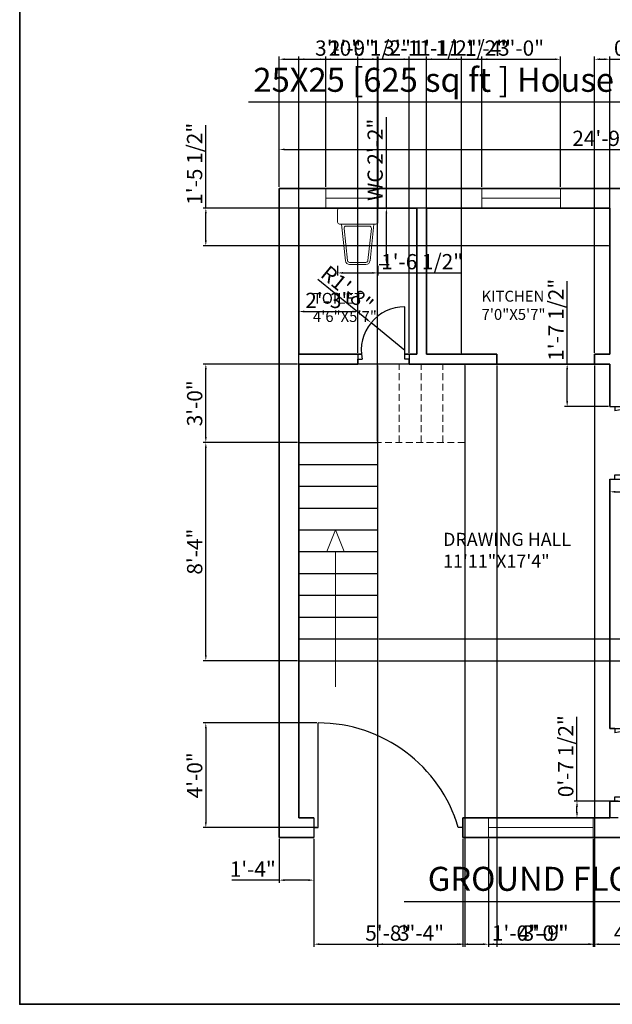
# Model space of a CAD drawing. Units: inches. Extents: x 1484 to 2008, y 1843 to 2590.
# Tile 1 of 21: x 1484 to 1756, y 1843 to 2295. Entities that reach past the tile are written whole.
import ezdxf

# ---------------------------------------------------------------- set-up
doc = ezdxf.new("R2010")
doc.units = ezdxf.units.IN
doc.linetypes.add('HIDDEN2', pattern=[4.7625, 3.175, -1.5875])
for name, color, linetype, lineweight in [('A-ANNO-DIMS', 2, 'Continuous', 18), ('A-ANNO-SYMB', 7, 'Continuous', 18), ('A-ANNO-TEXT', 7, 'Continuous', 25), ('A-ANNO-TTLB', 7, 'Continuous', 35), ('A-AREA-IDEN', 7, 'Continuous', 18), ('A-DOOR', 4, 'Continuous', 25), ('A-FLOR-FIXT', 9, 'Continuous', 18), ('A-FLOR-STRS', 7, 'Continuous', 25), ('A-FLOR-STRS-OVHD', 253, 'HIDDEN2', 18), ('A-GLAZ', 4, 'Continuous', 18), ('A-WALL', 7, 'Continuous', 35)]:
    doc.layers.add(name, color=color, linetype=linetype, lineweight=lineweight)
doc.styles.get("Standard").update_dxf_attribs({"font": 'arial.ttf'})
doc.dimstyles.new('ISO-25', dxfattribs={"dimtxt": 7, "dimasz": 2.5, "dimexe": 1.25, "dimexo": 0.625, "dimtad": 1, "dimdec": 0, "dimlunit": 3, "dimtxsty": 'Standard', "dimcen": 2.5, "dimadec": 0, "dimazin": 0, "dimtfac": 1, "dimtdec": 0, "dimtmove": 0, "dimatfit": 3, "dimfxl": 1, "dimarcsym": 0})

# ---------------------------------------------------------------- blocks, each defined once
blk = doc.blocks.new('A$C274B7A8C')
for p, q in [((0, 0.525), (0, 0.675)), ((0.025, 0.7), (0.475, 0.7)), ((0.5, 0.675), (0.5, 0.525)), ((0.475, 0.5), (0.025, 0.5)), ((0.05, 0.5), (0.098, 0.045)), ((0.402, 0.045), (0.45, 0.5)), ((0.081, 0.447), (0.123, 0.047)), ((0.106, 0.475), (0.394, 0.475)), ((0.377, 0.047), (0.419, 0.447)), ((0.148, 0.025), (0.352, 0.025)), ((0.148, 0), (0.352, 0))]:
    blk.add_line(p, q)
for centre, radius, start, end in [((0.025, 0.675), 0.025, 90, 180), ((0.475, 0.675), 0.025, 0, 90), ((0.025, 0.525), 0.025, 180, 270), ((0.475, 0.525), 0.025, 270, 0), ((0.106, 0.45), 0.025, 90, 186.009), ((0.394, 0.45), 0.025, 353.991, 90), ((0.148, 0.05), 0.05, 186.009, 270), ((0.148, 0.05), 0.025, 186.009, 270), ((0.352, 0.05), 0.025, 270, 353.991), ((0.352, 0.05), 0.05, 270, 353.991)]:
    blk.add_arc(centre, radius, start, end)
blk = doc.blocks.new('*D2')
at = {"layer": 'A-ANNO-DIMS', "color": 0, "lineweight": -2, "transparency": 16777216}
for p, q in [((1602.92, 2217.93), (1602.92, 2236.39)), ((1605.42, 2235.14), (1897.42, 2235.14)), ((1899.92, 2217.93), (1899.92, 2236.39))]:
    blk.add_line(p, q, dxfattribs=at)
at = {"layer": 'A-ANNO-DIMS', "color": 0, "transparency": 16777216}
for points in [[(1605.42, 2235.55), (1605.42, 2234.72), (1602.92, 2235.14)], [(1897.42, 2235.55), (1897.42, 2234.72), (1899.92, 2235.14)]]:
    blk.add_solid(points, dxfattribs=at)
at = {"layer": 'Defpoints', "color": 0, "transparency": 16777216}
for p in [(1899.92, 2235.14), (1602.92, 2217.3), (1899.92, 2217.3)]:
    blk.add_point(p, dxfattribs=at)
at = {"layer": 'A-ANNO-DIMS', "color": 0, "transparency": 16777216, "insert": (1750.41, 2239.33), "char_height": 7, "attachment_point": 5}
blk.add_mtext('24\'-9"', dxfattribs=at)
blk = doc.blocks.new('DOOR-SWING-36IN')
for p, q in [((-2.25, 31.33), (2.25, 31.33)), ((0, 31.33), (0, 29.33)), ((-2.25, -2), (2.25, -2)), ((0, -2), (0, 0)), ((0, 0), (36, 0))]:
    blk.add_line(p, q)
blk.add_arc((6.05, 0), 29.95, 0, 101.6643)
blk = doc.blocks.new('*D11')
at = {"layer": 'A-ANNO-DIMS', "color": 0, "lineweight": -2, "transparency": 16777216}
for p, q in [((1754.42, 2083.34), (1754.42, 2076.98)), ((1792.67, 2083.34), (1792.67, 2076.98)), ((1756.92, 2078.23), (1790.17, 2078.23)), ((1792.67, 2078.23), (1887.1, 2078.23))]:
    blk.add_line(p, q, dxfattribs=at)
at = {"layer": 'A-ANNO-DIMS', "color": 0, "transparency": 16777216}
for points in [[(1756.92, 2078.64), (1756.92, 2077.81), (1754.42, 2078.23)], [(1790.17, 2078.64), (1790.17, 2077.81), (1792.67, 2078.23)]]:
    blk.add_solid(points, dxfattribs=at)
at = {"layer": 'Defpoints', "color": 0, "transparency": 16777216}
for p in [(1754.42, 2083.96), (1792.67, 2083.96), (1792.67, 2078.23)]:
    blk.add_point(p, dxfattribs=at)
at = {"layer": 'A-ANNO-DIMS', "color": 0, "transparency": 16777216, "insert": (1841.14, 2082.47), "char_height": 7, "attachment_point": 5}
blk.add_mtext('DOOR 3\'-2 1/2" TYP.', dxfattribs=at)
blk = doc.blocks.new('*D17')
at = {"layer": 'A-ANNO-DIMS', "color": 0, "lineweight": -2, "transparency": 16777216}
for p, q in [((1652.04, 2208.3), (1652.04, 2249.96)), ((1648.78, 2208.3), (1653.29, 2208.3)), ((1652.04, 2184.93), (1652.04, 2205.8)), ((1648.78, 2182.43), (1653.29, 2182.43))]:
    blk.add_line(p, q, dxfattribs=at)
at = {"layer": 'A-ANNO-DIMS', "color": 0, "transparency": 16777216}
for points in [[(1651.62, 2205.8), (1652.46, 2205.8), (1652.04, 2208.3)], [(1651.62, 2184.93), (1652.46, 2184.93), (1652.04, 2182.43)]]:
    blk.add_solid(points, dxfattribs=at)
at = {"layer": 'Defpoints', "color": 0, "transparency": 16777216}
for p in [(1648.16, 2208.3), (1652.04, 2208.3), (1648.16, 2182.43)]:
    blk.add_point(p, dxfattribs=at)
at = {"layer": 'A-ANNO-DIMS', "color": 0, "transparency": 16777216, "insert": (1647.8, 2230.38), "char_height": 7, "attachment_point": 5, "rotation": 90}
blk.add_mtext('WC 2\'-2"', dxfattribs=at)
blk = doc.blocks.new('*D18')
at = {"layer": 'A-ANNO-DIMS', "color": 0, "lineweight": -2, "transparency": 16777216}
for p, q in [((1629.68, 2181.81), (1629.68, 2177.3)), ((1648.16, 2181.81), (1648.16, 2177.3)), ((1632.18, 2178.55), (1645.66, 2178.55)), ((1648.16, 2178.55), (1686.17, 2178.55))]:
    blk.add_line(p, q, dxfattribs=at)
at = {"layer": 'A-ANNO-DIMS', "color": 0, "transparency": 16777216}
for points in [[(1632.18, 2178.97), (1632.18, 2178.13), (1629.68, 2178.55)], [(1645.66, 2178.97), (1645.66, 2178.13), (1648.16, 2178.55)]]:
    blk.add_solid(points, dxfattribs=at)
at = {"layer": 'Defpoints', "color": 0, "transparency": 16777216}
for p in [(1629.68, 2182.43), (1648.16, 2182.43), (1648.16, 2178.55)]:
    blk.add_point(p, dxfattribs=at)
at = {"layer": 'A-ANNO-DIMS', "color": 0, "transparency": 16777216, "insert": (1668.41, 2182.79), "char_height": 7, "attachment_point": 5}
blk.add_mtext('1\'-6 1/2"', dxfattribs=at)
blk = doc.blocks.new('*D19')
at = {"layer": 'A-ANNO-DIMS', "color": 0, "lineweight": -2, "transparency": 16777216}
for p, q in [((1602.92, 1919.18), (1602.92, 1899)), ((1618.8, 1919.18), (1618.8, 1899)), ((1602.92, 1900.25), (1581.22, 1900.25)), ((1616.3, 1900.25), (1605.42, 1900.25))]:
    blk.add_line(p, q, dxfattribs=at)
at = {"layer": 'A-ANNO-DIMS', "color": 0, "transparency": 16777216}
for points in [[(1605.42, 1900.67), (1605.42, 1899.84), (1602.92, 1900.25)], [(1616.3, 1900.67), (1616.3, 1899.84), (1618.8, 1900.25)]]:
    blk.add_solid(points, dxfattribs=at)
at = {"layer": 'Defpoints', "color": 0, "transparency": 16777216}
for p in [(1602.92, 1919.8), (1618.8, 1919.8), (1602.92, 1900.25)]:
    blk.add_point(p, dxfattribs=at)
at = {"layer": 'A-ANNO-DIMS', "color": 0, "transparency": 16777216, "insert": (1590.82, 1904.39), "char_height": 7, "attachment_point": 5}
blk.add_mtext('1\'-4"', dxfattribs=at)
blk = doc.blocks.new('*D20')
at = {"layer": 'A-ANNO-DIMS', "color": 0, "lineweight": -2, "transparency": 16777216}
for p, q in [((1618.8, 1919.18), (1618.8, 1869.63)), ((1686.99, 1919.18), (1686.99, 1869.63)), ((1621.3, 1870.88), (1684.49, 1870.88))]:
    blk.add_line(p, q, dxfattribs=at)
at = {"layer": 'A-ANNO-DIMS', "color": 0, "transparency": 16777216}
for points in [[(1621.3, 1871.3), (1621.3, 1870.46), (1618.8, 1870.88)], [(1684.49, 1871.3), (1684.49, 1870.46), (1686.99, 1870.88)]]:
    blk.add_solid(points, dxfattribs=at)
at = {"layer": 'Defpoints', "color": 0, "transparency": 16777216}
for p in [(1618.8, 1919.8), (1686.99, 1919.8), (1686.99, 1870.88)]:
    blk.add_point(p, dxfattribs=at)
at = {"layer": 'A-ANNO-DIMS', "color": 0, "transparency": 16777216, "insert": (1652.89, 1875.08), "char_height": 7, "attachment_point": 5}
blk.add_mtext('5\'-8"', dxfattribs=at)
blk = doc.blocks.new('*D21')
at = {"layer": 'A-ANNO-DIMS', "color": 0, "lineweight": -2, "transparency": 16777216}
for p, q in [((1686.99, 1919.18), (1686.99, 1869.63)), ((1698.84, 1919.18), (1698.84, 1869.63)), ((1689.49, 1870.88), (1696.34, 1870.88)), ((1698.84, 1870.88), (1720.54, 1870.88))]:
    blk.add_line(p, q, dxfattribs=at)
at = {"layer": 'A-ANNO-DIMS', "color": 0, "transparency": 16777216}
for points in [[(1689.49, 1871.3), (1689.49, 1870.46), (1686.99, 1870.88)], [(1696.34, 1871.3), (1696.34, 1870.46), (1698.84, 1870.88)]]:
    blk.add_solid(points, dxfattribs=at)
at = {"layer": 'Defpoints', "color": 0, "transparency": 16777216}
for p in [(1686.99, 1919.8), (1698.84, 1919.8), (1698.84, 1870.88)]:
    blk.add_point(p, dxfattribs=at)
at = {"layer": 'A-ANNO-DIMS', "color": 0, "transparency": 16777216, "insert": (1710.94, 1875.08), "char_height": 7, "attachment_point": 5}
blk.add_mtext('1\'-0"', dxfattribs=at)
blk = doc.blocks.new('*D22')
at = {"layer": 'A-ANNO-DIMS', "color": 0, "lineweight": -2, "transparency": 16777216}
for p, q in [((1698.84, 1919.18), (1698.84, 1869.63)), ((1746.84, 1919.18), (1746.84, 1869.63)), ((1701.34, 1870.88), (1744.34, 1870.88))]:
    blk.add_line(p, q, dxfattribs=at)
at = {"layer": 'A-ANNO-DIMS', "color": 0, "transparency": 16777216}
for points in [[(1701.34, 1871.3), (1701.34, 1870.46), (1698.84, 1870.88)], [(1744.34, 1871.3), (1744.34, 1870.46), (1746.84, 1870.88)]]:
    blk.add_solid(points, dxfattribs=at)
at = {"layer": 'Defpoints', "color": 0, "transparency": 16777216}
for p in [(1698.84, 1919.8), (1746.84, 1919.8), (1746.84, 1870.88)]:
    blk.add_point(p, dxfattribs=at)
at = {"layer": 'A-ANNO-DIMS', "color": 0, "transparency": 16777216, "insert": (1722.84, 1875.08), "char_height": 7, "attachment_point": 5}
blk.add_mtext('4\'-0"', dxfattribs=at)
blk = doc.blocks.new('*D23')
at = {"layer": 'A-ANNO-DIMS', "color": 0, "lineweight": -2, "transparency": 16777216}
for p, q in [((1746.84, 1919.18), (1746.84, 1869.63)), ((1803.22, 1919.18), (1803.22, 1869.63)), ((1749.34, 1870.88), (1800.72, 1870.88))]:
    blk.add_line(p, q, dxfattribs=at)
at = {"layer": 'A-ANNO-DIMS', "color": 0, "transparency": 16777216}
for points in [[(1749.34, 1871.3), (1749.34, 1870.46), (1746.84, 1870.88)], [(1800.72, 1871.3), (1800.72, 1870.46), (1803.22, 1870.88)]]:
    blk.add_solid(points, dxfattribs=at)
at = {"layer": 'Defpoints', "color": 0, "transparency": 16777216}
for p in [(1746.84, 1919.8), (1803.22, 1919.8), (1803.22, 1870.88)]:
    blk.add_point(p, dxfattribs=at)
at = {"layer": 'A-ANNO-DIMS', "color": 0, "transparency": 16777216, "insert": (1775.03, 1875.12), "char_height": 7, "attachment_point": 5}
blk.add_mtext('4\'-8 1/2"', dxfattribs=at)
blk = doc.blocks.new('*D24')
at = {"layer": 'A-ANNO-DIMS', "color": 0, "lineweight": -2, "transparency": 16777216}
for p, q in [((1602.92, 2217.93), (1602.92, 2277.72)), ((1605.42, 2276.47), (1621.73, 2276.47)), ((1624.23, 2217.93), (1624.23, 2277.72)), ((1624.23, 2276.47), (1662.24, 2276.47))]:
    blk.add_line(p, q, dxfattribs=at)
at = {"layer": 'A-ANNO-DIMS', "color": 0, "transparency": 16777216}
for points in [[(1605.42, 2276.89), (1605.42, 2276.06), (1602.92, 2276.47)], [(1621.73, 2276.89), (1621.73, 2276.06), (1624.23, 2276.47)]]:
    blk.add_solid(points, dxfattribs=at)
at = {"layer": 'Defpoints', "color": 0, "transparency": 16777216}
for p in [(1624.23, 2276.47), (1602.92, 2217.3), (1624.23, 2217.3)]:
    blk.add_point(p, dxfattribs=at)
at = {"layer": 'A-ANNO-DIMS', "color": 0, "transparency": 16777216, "insert": (1644.48, 2280.72), "char_height": 7, "attachment_point": 5}
blk.add_mtext('1\'-9 1/2"', dxfattribs=at)
blk = doc.blocks.new('*D25')
at = {"layer": 'A-ANNO-DIMS', "color": 0, "lineweight": -2, "transparency": 16777216}
for p, q in [((1624.23, 2217.93), (1624.23, 2277.72)), ((1626.73, 2276.47), (1645.73, 2276.47)), ((1648.23, 2217.93), (1648.23, 2277.72))]:
    blk.add_line(p, q, dxfattribs=at)
at = {"layer": 'A-ANNO-DIMS', "color": 0, "transparency": 16777216}
for points in [[(1626.73, 2276.89), (1626.73, 2276.06), (1624.23, 2276.47)], [(1645.73, 2276.89), (1645.73, 2276.06), (1648.23, 2276.47)]]:
    blk.add_solid(points, dxfattribs=at)
at = {"layer": 'Defpoints', "color": 0, "transparency": 16777216}
for p in [(1648.23, 2276.47), (1624.23, 2217.3), (1648.23, 2217.3)]:
    blk.add_point(p, dxfattribs=at)
at = {"layer": 'A-ANNO-DIMS', "color": 0, "transparency": 16777216, "insert": (1636.23, 2280.67), "char_height": 7, "attachment_point": 5}
blk.add_mtext('2\'-0"', dxfattribs=at)
blk = doc.blocks.new('*D26')
at = {"layer": 'A-ANNO-DIMS', "color": 0, "lineweight": -2, "transparency": 16777216}
for p, q in [((1648.23, 2217.93), (1648.23, 2277.72)), ((1650.73, 2276.47), (1693.24, 2276.47)), ((1695.74, 2217.93), (1695.74, 2277.72))]:
    blk.add_line(p, q, dxfattribs=at)
at = {"layer": 'A-ANNO-DIMS', "color": 0, "transparency": 16777216}
for points in [[(1650.73, 2276.89), (1650.73, 2276.06), (1648.23, 2276.47)], [(1693.24, 2276.89), (1693.24, 2276.06), (1695.74, 2276.47)]]:
    blk.add_solid(points, dxfattribs=at)
at = {"layer": 'Defpoints', "color": 0, "transparency": 16777216}
for p in [(1695.74, 2276.47), (1648.23, 2217.3), (1695.74, 2217.3)]:
    blk.add_point(p, dxfattribs=at)
at = {"layer": 'A-ANNO-DIMS', "color": 0, "transparency": 16777216, "insert": (1671.98, 2280.72), "char_height": 7, "attachment_point": 5}
blk.add_mtext('3\'-11 1/2"', dxfattribs=at)
blk = doc.blocks.new('*D27')
at = {"layer": 'A-ANNO-DIMS', "color": 0, "lineweight": -2, "transparency": 16777216}
for p, q in [((1695.74, 2217.93), (1695.74, 2277.72)), ((1698.24, 2276.47), (1729.24, 2276.47)), ((1731.74, 2217.93), (1731.74, 2277.72))]:
    blk.add_line(p, q, dxfattribs=at)
at = {"layer": 'A-ANNO-DIMS', "color": 0, "transparency": 16777216}
for points in [[(1698.24, 2276.89), (1698.24, 2276.06), (1695.74, 2276.47)], [(1729.24, 2276.89), (1729.24, 2276.06), (1731.74, 2276.47)]]:
    blk.add_solid(points, dxfattribs=at)
at = {"layer": 'Defpoints', "color": 0, "transparency": 16777216}
for p in [(1731.74, 2276.47), (1695.74, 2217.3), (1731.74, 2217.3)]:
    blk.add_point(p, dxfattribs=at)
at = {"layer": 'A-ANNO-DIMS', "color": 0, "transparency": 16777216, "insert": (1713.74, 2280.68), "char_height": 7, "attachment_point": 5}
blk.add_mtext('3\'-0"', dxfattribs=at)
blk = doc.blocks.new('*D29')
at = {"layer": 'A-ANNO-DIMS', "color": 0, "lineweight": -2, "transparency": 16777216}
for p, q in [((1620.17, 1972.3), (1568.06, 1972.3)), ((1569.31, 1969.8), (1569.31, 1926.8)), ((1620.17, 1924.3), (1568.06, 1924.3))]:
    blk.add_line(p, q, dxfattribs=at)
at = {"layer": 'A-ANNO-DIMS', "color": 0, "transparency": 16777216}
for points in [[(1568.9, 1969.8), (1569.73, 1969.8), (1569.31, 1972.3)], [(1568.9, 1926.8), (1569.73, 1926.8), (1569.31, 1924.3)]]:
    blk.add_solid(points, dxfattribs=at)
at = {"layer": 'Defpoints', "color": 0, "transparency": 16777216}
for p in [(1620.8, 1972.3), (1569.31, 1924.3), (1620.8, 1924.3)]:
    blk.add_point(p, dxfattribs=at)
at = {"layer": 'A-ANNO-DIMS', "color": 0, "transparency": 16777216, "insert": (1565.11, 1948.3), "char_height": 7, "attachment_point": 5, "rotation": 90}
blk.add_mtext('4\'-0"', dxfattribs=at)
blk = doc.blocks.new('*D30')
at = {"layer": 'A-ANNO-DIMS', "color": 0, "lineweight": -2, "transparency": 16777216}
for p, q in [((1611.92, 2101.43), (1611.92, 2277.72)), ((1614.42, 2276.47), (1645.42, 2276.47)), ((1647.92, 2101.43), (1647.92, 2277.72))]:
    blk.add_line(p, q, dxfattribs=at)
at = {"layer": 'A-ANNO-DIMS', "color": 0, "transparency": 16777216}
for points in [[(1614.42, 2276.89), (1614.42, 2276.06), (1611.92, 2276.47)], [(1645.42, 2276.89), (1645.42, 2276.06), (1647.92, 2276.47)]]:
    blk.add_solid(points, dxfattribs=at)
at = {"layer": 'Defpoints', "color": 0, "transparency": 16777216}
for p in [(1647.92, 2276.47), (1611.92, 2100.8), (1647.92, 2100.8)]:
    blk.add_point(p, dxfattribs=at)
at = {"layer": 'A-ANNO-DIMS', "color": 0, "transparency": 16777216, "insert": (1629.92, 2280.68), "char_height": 7, "attachment_point": 5}
blk.add_mtext('3\'-0"', dxfattribs=at)
blk = doc.blocks.new('*D31')
at = {"layer": 'A-ANNO-DIMS', "color": 0, "lineweight": -2, "transparency": 16777216}
for p, q in [((1611.29, 2100.8), (1568.06, 2100.8)), ((1569.31, 2003.3), (1569.31, 2098.3)), ((1611.29, 2000.8), (1568.06, 2000.8))]:
    blk.add_line(p, q, dxfattribs=at)
at = {"layer": 'A-ANNO-DIMS', "color": 0, "transparency": 16777216}
for points in [[(1568.9, 2098.3), (1569.73, 2098.3), (1569.31, 2100.8)], [(1568.9, 2003.3), (1569.73, 2003.3), (1569.31, 2000.8)]]:
    blk.add_solid(points, dxfattribs=at)
at = {"layer": 'Defpoints', "color": 0, "transparency": 16777216}
for p in [(1569.31, 2100.8), (1611.92, 2100.8), (1611.92, 2000.8)]:
    blk.add_point(p, dxfattribs=at)
at = {"layer": 'A-ANNO-DIMS', "color": 0, "transparency": 16777216, "insert": (1565.11, 2050.8), "char_height": 7, "attachment_point": 5, "rotation": 90}
blk.add_mtext('8\'-4"', dxfattribs=at)
blk = doc.blocks.new('*D32')
at = {"layer": 'A-ANNO-DIMS', "color": 0, "lineweight": -2, "transparency": 16777216}
for p, q in [((1961.85, 2010.8), (1961.85, 2038.6)), ((1648.54, 2010.8), (1963.1, 2010.8)), ((1961.85, 2003.3), (1961.85, 2008.3)), ((1648.54, 2000.8), (1963.1, 2000.8))]:
    blk.add_line(p, q, dxfattribs=at)
at = {"layer": 'A-ANNO-DIMS', "color": 0, "transparency": 16777216}
for points in [[(1961.44, 2008.3), (1962.27, 2008.3), (1961.85, 2010.8)], [(1961.44, 2003.3), (1962.27, 2003.3), (1961.85, 2000.8)]]:
    blk.add_solid(points, dxfattribs=at)
at = {"layer": 'Defpoints', "color": 0, "transparency": 16777216}
for p in [(1647.92, 2010.8), (1961.85, 2010.8), (1647.92, 2000.8)]:
    blk.add_point(p, dxfattribs=at)
at = {"layer": 'A-ANNO-DIMS', "color": 0, "transparency": 16777216, "insert": (1957.66, 2025.95), "char_height": 7, "attachment_point": 5, "rotation": 90}
blk.add_mtext('0\'-10"', dxfattribs=at)
blk = doc.blocks.new('*D33')
at = {"layer": 'A-ANNO-DIMS', "color": 0, "lineweight": -2, "transparency": 16777216}
for p, q in [((1611.29, 2136.8), (1568.06, 2136.8)), ((1569.31, 2103.3), (1569.31, 2134.3)), ((1611.29, 2100.8), (1568.06, 2100.8))]:
    blk.add_line(p, q, dxfattribs=at)
at = {"layer": 'A-ANNO-DIMS', "color": 0, "transparency": 16777216}
for points in [[(1568.9, 2134.3), (1569.73, 2134.3), (1569.31, 2136.8)], [(1568.9, 2103.3), (1569.73, 2103.3), (1569.31, 2100.8)]]:
    blk.add_solid(points, dxfattribs=at)
at = {"layer": 'Defpoints', "color": 0, "transparency": 16777216}
for p in [(1569.31, 2136.8), (1611.92, 2136.8), (1611.92, 2100.8)]:
    blk.add_point(p, dxfattribs=at)
at = {"layer": 'A-ANNO-DIMS', "color": 0, "transparency": 16777216, "insert": (1565.11, 2118.8), "char_height": 7, "attachment_point": 5, "rotation": 90}
blk.add_mtext('3\'-0"', dxfattribs=at)
blk = doc.blocks.new('*D34')
at = {"layer": 'A-ANNO-DIMS', "color": 0, "lineweight": -2, "transparency": 16777216}
for p, q in [((1647.92, 2136.18), (1647.92, 1869.63)), ((1687.92, 2136.18), (1687.92, 1869.63)), ((1650.42, 1870.88), (1685.42, 1870.88))]:
    blk.add_line(p, q, dxfattribs=at)
at = {"layer": 'A-ANNO-DIMS', "color": 0, "transparency": 16777216}
for points in [[(1650.42, 1871.3), (1650.42, 1870.46), (1647.92, 1870.88)], [(1685.42, 1871.3), (1685.42, 1870.46), (1687.92, 1870.88)]]:
    blk.add_solid(points, dxfattribs=at)
at = {"layer": 'Defpoints', "color": 0, "transparency": 16777216}
for p in [(1647.92, 2136.8), (1687.92, 2136.8), (1687.92, 1870.88)]:
    blk.add_point(p, dxfattribs=at)
at = {"layer": 'A-ANNO-DIMS', "color": 0, "transparency": 16777216, "insert": (1667.92, 1875.08), "char_height": 7, "attachment_point": 5}
blk.add_mtext('3\'-4"', dxfattribs=at)
blk = doc.blocks.new('*D35')
at = {"layer": 'A-ANNO-DIMS', "color": 0, "lineweight": -2, "transparency": 16777216}
for p, q in [((1638.92, 2141.93), (1638.92, 2277.72)), ((1641.42, 2276.47), (1660.01, 2276.47)), ((1662.51, 2141.93), (1662.51, 2277.72)), ((1662.51, 2276.47), (1705.96, 2276.47))]:
    blk.add_line(p, q, dxfattribs=at)
at = {"layer": 'A-ANNO-DIMS', "color": 0, "transparency": 16777216}
for points in [[(1641.42, 2276.89), (1641.42, 2276.06), (1638.92, 2276.47)], [(1660.01, 2276.89), (1660.01, 2276.06), (1662.51, 2276.47)]]:
    blk.add_solid(points, dxfattribs=at)
at = {"layer": 'Defpoints', "color": 0, "transparency": 16777216}
for p in [(1662.51, 2276.47), (1638.92, 2141.3), (1662.51, 2141.3)]:
    blk.add_point(p, dxfattribs=at)
at = {"layer": 'A-ANNO-DIMS', "color": 0, "transparency": 16777216, "insert": (1685.48, 2280.72), "char_height": 7, "attachment_point": 5}
blk.add_mtext('1\'-11 1/2"', dxfattribs=at)
blk = doc.blocks.new('*D36')
at = {"layer": 'A-ANNO-DIMS', "color": 0, "lineweight": -2, "transparency": 16777216}
for p, q in [((1611.92, 2141.93), (1611.92, 2162.1)), ((1638.92, 2141.93), (1638.92, 2162.1)), ((1614.42, 2160.85), (1636.42, 2160.85))]:
    blk.add_line(p, q, dxfattribs=at)
at = {"layer": 'A-ANNO-DIMS', "color": 0, "transparency": 16777216}
for points in [[(1614.42, 2161.27), (1614.42, 2160.44), (1611.92, 2160.85)], [(1636.42, 2161.27), (1636.42, 2160.44), (1638.92, 2160.85)]]:
    blk.add_solid(points, dxfattribs=at)
at = {"layer": 'Defpoints', "color": 0, "transparency": 16777216}
for p in [(1638.92, 2160.85), (1611.92, 2141.3), (1638.92, 2141.3)]:
    blk.add_point(p, dxfattribs=at)
at = {"layer": 'A-ANNO-DIMS', "color": 0, "transparency": 16777216, "insert": (1625.42, 2165.05), "char_height": 7, "attachment_point": 5}
blk.add_mtext('2\'-3"', dxfattribs=at)
blk = doc.blocks.new('*D37')
at = {"layer": 'A-ANNO-DIMS', "color": 0, "lineweight": -2, "transparency": 16777216}
for p, q in [((1702.57, 2136.18), (1702.57, 1869.63)), ((1747.43, 2136.18), (1747.43, 1869.63)), ((1705.07, 1870.88), (1744.93, 1870.88))]:
    blk.add_line(p, q, dxfattribs=at)
at = {"layer": 'A-ANNO-DIMS', "color": 0, "transparency": 16777216}
for points in [[(1705.07, 1871.3), (1705.07, 1870.46), (1702.57, 1870.88)], [(1744.93, 1871.3), (1744.93, 1870.46), (1747.43, 1870.88)]]:
    blk.add_solid(points, dxfattribs=at)
at = {"layer": 'Defpoints', "color": 0, "transparency": 16777216}
for p in [(1702.57, 2136.8), (1747.43, 2136.8), (1747.43, 1870.88)]:
    blk.add_point(p, dxfattribs=at)
at = {"layer": 'A-ANNO-DIMS', "color": 0, "transparency": 16777216, "insert": (1725, 1875.08), "char_height": 7, "attachment_point": 5}
blk.add_mtext('3\'-9"', dxfattribs=at)
blk = doc.blocks.new('*D38')
at = {"layer": 'A-ANNO-DIMS', "color": 0, "lineweight": -2, "transparency": 16777216}
for p, q in [((1747.43, 2141.93), (1747.43, 2277.72)), ((1749.93, 2276.47), (1751.92, 2276.47)), ((1754.42, 2141.93), (1754.42, 2277.72)), ((1754.42, 2276.47), (1776.78, 2276.47))]:
    blk.add_line(p, q, dxfattribs=at)
at = {"layer": 'A-ANNO-DIMS', "color": 0, "transparency": 16777216}
for points in [[(1749.93, 2276.89), (1749.93, 2276.06), (1747.43, 2276.47)], [(1751.92, 2276.89), (1751.92, 2276.06), (1754.42, 2276.47)]]:
    blk.add_solid(points, dxfattribs=at)
at = {"layer": 'Defpoints', "color": 0, "transparency": 16777216}
for p in [(1754.42, 2276.47), (1747.43, 2141.3), (1754.42, 2141.3)]:
    blk.add_point(p, dxfattribs=at)
at = {"layer": 'A-ANNO-DIMS', "color": 0, "transparency": 16777216, "insert": (1766.85, 2280.67), "char_height": 7, "attachment_point": 5}
blk.add_mtext('0\'-7"', dxfattribs=at)
blk = doc.blocks.new('*D39')
at = {"layer": 'A-ANNO-DIMS', "color": 0, "lineweight": -2, "transparency": 16777216}
for p, q in [((1734.87, 2136.8), (1734.87, 2174.81)), ((1753.79, 2136.8), (1733.62, 2136.8)), ((1734.87, 2119.79), (1734.87, 2134.3)), ((1753.79, 2117.29), (1733.62, 2117.29))]:
    blk.add_line(p, q, dxfattribs=at)
at = {"layer": 'A-ANNO-DIMS', "color": 0, "transparency": 16777216}
for points in [[(1734.45, 2134.3), (1735.29, 2134.3), (1734.87, 2136.8)], [(1734.45, 2119.79), (1735.29, 2119.79), (1734.87, 2117.29)]]:
    blk.add_solid(points, dxfattribs=at)
at = {"layer": 'Defpoints', "color": 0, "transparency": 16777216}
for p in [(1734.87, 2136.8), (1754.42, 2136.8), (1754.42, 2117.29)]:
    blk.add_point(p, dxfattribs=at)
at = {"layer": 'A-ANNO-DIMS', "color": 0, "transparency": 16777216, "insert": (1730.63, 2157.06), "char_height": 7, "attachment_point": 5, "rotation": 90}
blk.add_mtext('1\'-7 1/2"', dxfattribs=at)
blk = doc.blocks.new('*D40')
at = {"layer": 'A-ANNO-DIMS', "color": 0, "lineweight": -2, "transparency": 16777216}
for p, q in [((1739.37, 1936.47), (1739.37, 1975.14)), ((1758.29, 1936.47), (1738.12, 1936.47)), ((1739.37, 1931.3), (1739.37, 1933.97)), ((1758.29, 1928.8), (1738.12, 1928.8))]:
    blk.add_line(p, q, dxfattribs=at)
at = {"layer": 'A-ANNO-DIMS', "color": 0, "transparency": 16777216}
for points in [[(1738.95, 1933.97), (1739.79, 1933.97), (1739.37, 1936.47)], [(1738.95, 1931.3), (1739.79, 1931.3), (1739.37, 1928.8)]]:
    blk.add_solid(points, dxfattribs=at)
at = {"layer": 'Defpoints', "color": 0, "transparency": 16777216}
for p in [(1739.37, 1936.47), (1758.92, 1936.47), (1758.92, 1928.8)]:
    blk.add_point(p, dxfattribs=at)
at = {"layer": 'A-ANNO-DIMS', "color": 0, "transparency": 16777216, "insert": (1735.13, 1957.05), "char_height": 7, "attachment_point": 5, "rotation": 90}
blk.add_mtext('0\'-7 1/2"', dxfattribs=at)
blk = doc.blocks.new('*D42')
at = {"layer": 'A-ANNO-DIMS', "color": 0, "lineweight": -2, "transparency": 16777216}
for p, q in [((1670.42, 2141.93), (1670.42, 2277.72)), ((1672.92, 2276.47), (1684, 2276.47)), ((1686.5, 2141.93), (1686.5, 2277.72)), ((1686.5, 2276.47), (1708.19, 2276.47))]:
    blk.add_line(p, q, dxfattribs=at)
at = {"layer": 'A-ANNO-DIMS', "color": 0, "transparency": 16777216}
for points in [[(1672.92, 2276.89), (1672.92, 2276.06), (1670.42, 2276.47)], [(1684, 2276.89), (1684, 2276.06), (1686.5, 2276.47)]]:
    blk.add_solid(points, dxfattribs=at)
at = {"layer": 'Defpoints', "color": 0, "transparency": 16777216}
for p in [(1686.5, 2276.47), (1670.42, 2141.3), (1686.5, 2141.3)]:
    blk.add_point(p, dxfattribs=at)
at = {"layer": 'A-ANNO-DIMS', "color": 0, "transparency": 16777216, "insert": (1698.6, 2280.61), "char_height": 7, "attachment_point": 5}
blk.add_mtext('1\'-4"', dxfattribs=at)
blk = doc.blocks.new('*D43')
at = {"layer": 'A-ANNO-DIMS', "color": 0, "lineweight": -2, "transparency": 16777216}
for p, q in [((1569.31, 2208.3), (1569.31, 2246.31)), ((1753.79, 2208.3), (1568.06, 2208.3)), ((1569.31, 2193.46), (1569.31, 2205.8)), ((1753.79, 2190.96), (1568.06, 2190.96))]:
    blk.add_line(p, q, dxfattribs=at)
at = {"layer": 'A-ANNO-DIMS', "color": 0, "transparency": 16777216}
for points in [[(1568.9, 2205.8), (1569.73, 2205.8), (1569.31, 2208.3)], [(1568.9, 2193.46), (1569.73, 2193.46), (1569.31, 2190.96)]]:
    blk.add_solid(points, dxfattribs=at)
at = {"layer": 'Defpoints', "color": 0, "transparency": 16777216}
for p in [(1569.31, 2208.3), (1754.42, 2208.3), (1754.42, 2190.96)]:
    blk.add_point(p, dxfattribs=at)
at = {"layer": 'A-ANNO-DIMS', "color": 0, "transparency": 16777216, "insert": (1565.07, 2228.56), "char_height": 7, "attachment_point": 5, "rotation": 90}
blk.add_mtext('1\'-5 1/2"', dxfattribs=at)
blk = doc.blocks.new('*D66')
at = {"layer": 'A-ANNO-DIMS', "color": 0, "lineweight": -2, "transparency": 16777216}
for p, q in [((1620.57, 2175.65), (1643.08, 2157.28)), ((1660.51, 2143.06), (1645.02, 2155.7))]:
    blk.add_line(p, q, dxfattribs=at)
at = {"layer": 'A-ANNO-DIMS', "color": 0, "transparency": 16777216}
blk.add_solid([(1643.34, 2157.6), (1642.82, 2156.96), (1645.02, 2155.7)], dxfattribs=at)
at = {"layer": 'Defpoints', "color": 0, "transparency": 16777216}
for p in [(1645.02, 2155.7), (1660.51, 2143.06)]:
    blk.add_point(p, dxfattribs=at)
at = {"layer": 'A-ANNO-DIMS', "color": 0, "transparency": 16777216, "insert": (1633.51, 2170.51), "char_height": 7, "attachment_point": 5, "rotation": 320.7808}
blk.add_mtext('R1\'-8"', dxfattribs=at)

msp = doc.modelspace()

# ---------------------------------------------------------------- linework, layer by layer
at = {"layer": 'A-ANNO-SYMB'}
for p, q in [((1628.72, 2060.8), (1624.72, 2050.8)), ((1632.63, 2050.8), (1628.72, 2060.8)), ((1624.72, 2050.8), (1632.63, 2050.8)), ((1628.72, 1988.79), (1628.72, 2050.8))]:
    msp.add_line(p, q, dxfattribs=at)
at = {"layer": 'A-ANNO-TEXT'}
for p, q in [((1588.86, 2256.92), (1942.3, 2256.92)), ((1660.24, 1890.43), (1846.57, 1890.43))]:
    msp.add_line(p, q, dxfattribs=at)
at = {"layer": 'A-ANNO-TTLB'}
msp.add_lwpolyline([(1484.04, 2590.09), (1989.53, 2590.09), (1989.53, 1843.34), (1484.04, 1843.34)], close=True, dxfattribs=at)
at = {"layer": 'A-DOOR'}
for p, q in [((1660.51, 2139.05), (1660.51, 2163.05)), ((1638.92, 2141.3), (1638.92, 2136.8)), ((1638.92, 2136.8), (1638.92, 2139.05)), ((1638.92, 2139.05), (1640.92, 2139.05)), ((1662.51, 2139.05), (1660.51, 2139.05)), ((1662.51, 2141.3), (1662.51, 2136.8)), ((1662.51, 2136.8), (1662.51, 2139.05)), ((1662.51, 2136.8), (1638.92, 2136.8)), ((1620.8, 1924.3), (1620.8, 1972.3)), ((1756.67, 1969.8), (1754.42, 1969.8)), ((1618.8, 1928.8), (1618.8, 1919.8)), ((1683.17, 1928.8), (1683.17, 1928.8)), ((1686.99, 1928.8), (1686.99, 1919.8)), ((1686.99, 1919.8), (1686.99, 1928.8)), ((1618.8, 1924.3), (1620.8, 1924.3)), ((1686.99, 1924.3), (1684.99, 1924.3))]:
    msp.add_line(p, q, dxfattribs=at)
for centre, radius, start, end in [((1660.51, 2143.06), 19.99, 90, 191.5596), ((1620.8, 1905.37), 66.93, 16.4292, 90)]:
    msp.add_arc(centre, radius, start, end, dxfattribs=at)
at = {"layer": 'A-FLOR-FIXT'}
for p, q in [((1686.5, 2141.3), (1686.5, 2190.96)), ((1686.5, 2190.96), (1754.42, 2190.96))]:
    msp.add_line(p, q, dxfattribs=at)
at = {"layer": 'A-FLOR-STRS'}
for p, q in [((1611.92, 2136.8), (1611.92, 2100.8)), ((1611.92, 2100.8), (1647.92, 2100.8)), ((1647.92, 2100.8), (1647.92, 2000.8)), ((1611.92, 2090.8), (1647.92, 2090.8)), ((1611.92, 2080.8), (1647.92, 2080.8)), ((1611.92, 2070.8), (1647.92, 2070.8)), ((1611.92, 2060.8), (1647.92, 2060.8)), ((1611.92, 2050.8), (1647.92, 2050.8)), ((1611.92, 2040.8), (1647.92, 2040.8)), ((1611.92, 2030.8), (1647.92, 2030.8)), ((1611.92, 2020.8), (1647.92, 2020.8)), ((1611.92, 2010.8), (1647.92, 2010.8)), ((1611.92, 2000.8), (1647.92, 2000.8))]:
    msp.add_line(p, q, dxfattribs=at)
at = {"layer": 'A-FLOR-STRS-OVHD'}
for p, q in [((1647.92, 2100.8), (1647.92, 2136.8)), ((1657.92, 2100.8), (1657.92, 2136.8)), ((1667.92, 2100.8), (1667.92, 2136.8)), ((1677.92, 2100.8), (1677.92, 2136.8)), ((1687.92, 2100.8), (1687.92, 2136.8)), ((1687.92, 2100.8), (1647.92, 2100.8))]:
    msp.add_line(p, q, dxfattribs=at)
at = {"layer": 'A-GLAZ'}
for p, q in [((1624.23, 2217.3), (1624.23, 2208.3)), ((1648.23, 2212.8), (1648.23, 2217.3)), ((1648.23, 2217.3), (1648.23, 2208.3)), ((1695.74, 2208.3), (1695.74, 2217.3)), ((1695.74, 2217.3), (1695.74, 2212.8)), ((1731.74, 2212.8), (1731.74, 2217.3)), ((1731.74, 2217.3), (1731.74, 2208.3)), ((1624.23, 2208.3), (1624.23, 2212.8)), ((1624.23, 2212.8), (1648.23, 2212.8)), ((1695.74, 2212.8), (1731.74, 2212.8)), ((1698.84, 1924.3), (1698.84, 1928.8)), ((1698.84, 1928.8), (1698.84, 1919.8)), ((1746.84, 1928.8), (1746.84, 1919.8)), ((1746.84, 1924.3), (1698.84, 1924.3)), ((1746.84, 1919.8), (1746.84, 1924.3))]:
    msp.add_line(p, q, dxfattribs=at)
at = {"layer": 'A-WALL'}
for p, q in [((1602.92, 2217.3), (1602.92, 1919.8)), ((1602.92, 2217.3), (1899.92, 2217.3)), ((1602.92, 2217.3), (1899.92, 2217.3)), ((1611.92, 2208.3), (1665.92, 2208.3)), ((1611.92, 2208.3), (1611.92, 2141.3)), ((1665.92, 2208.3), (1665.92, 2141.3)), ((1670.42, 2208.3), (1670.42, 2141.3)), ((1670.42, 2208.3), (1754.42, 2208.3)), ((1754.42, 2208.3), (1754.42, 2141.3)), ((1611.92, 2141.3), (1640.59, 2141.3)), ((1660.51, 2141.3), (1665.92, 2141.3)), ((1670.42, 2141.3), (1702.57, 2141.3)), ((1702.57, 2141.3), (1702.57, 2136.8)), ((1747.43, 2141.3), (1747.43, 2136.8)), ((1747.43, 2141.3), (1754.42, 2141.3)), ((1611.92, 2136.8), (1638.92, 2136.8)), ((1611.92, 2136.8), (1611.92, 1928.8)), ((1662.51, 2136.8), (1754.42, 2136.8)), ((1754.42, 2136.8), (1754.42, 2117.29)), ((1754.42, 2083.96), (1754.42, 1969.8)), ((1754.42, 1936.47), (1754.42, 1928.8)), ((1611.92, 1928.8), (1618.8, 1928.8)), ((1686.99, 1928.8), (1754.42, 1928.8)), ((1602.92, 1919.8), (1618.8, 1919.8)), ((1686.99, 1919.8), (1899.92, 1919.8))]:
    msp.add_line(p, q, dxfattribs=at)

# ---------------------------------------------------------------- block references
at = {"layer": 'A-DOOR'}
for p in [(1756.67, 2085.96), (1756.67, 1938.47)]:
    msp.add_blockref('DOOR-SWING-36IN', p, dxfattribs=at)
at = {"layer": 'A-FLOR-FIXT', "xscale": 36.95985685062697, "yscale": 36.95985685062697, "zscale": 36.95985685062697}
msp.add_blockref('A$C274B7A8C', (1629.68, 2182.43), dxfattribs=at)

# ---------------------------------------------------------------- texts
at = {"layer": 'A-ANNO-TEXT', "char_height": 11, "attachment_point": 1}
for s, width, insert in [('25X25 [625 sq ft ] House Plan -North face - FP1321', 378.3718, (1591.11, 2272.55)), ('GROUND FLOOR PLAN', 211.2221, (1671, 1906.35))]:
    msp.add_mtext_dynamic_manual_height_columns(s, width=width, gutter_width=12.5, heights=[0], dxfattribs=dict(at, insert=insert))
at = {"layer": 'A-AREA-IDEN', "attachment_point": 1}
for s, width, insert, char_height in [('TOILET\\P4\'6"X5\'7"', 38.1947, (1618.38, 2169.41), 5), ('KITCHEN\\P7\'0"X5\'7"', 54.8732, (1695.64, 2170.37), 5), ('DRAWING HALL\\P11\'11"X17\'4"', 96.872, (1678.03, 2059.43), 6)]:
    msp.add_mtext_dynamic_manual_height_columns(s, width=width, gutter_width=12.5, heights=[0], dxfattribs=dict(at, insert=insert, char_height=char_height))

# ---------------------------------------------------------------- dimensions: what is measured, and where the dimension line sits
at = {"layer": 'A-ANNO-DIMS'}
for base, p1, p2, picture, middle in [((1624.23, 2276.47), (1602.92, 2217.3), (1624.23, 2217.3), '*D24', (1644.48, 2280.72)), ((1662.51, 2276.47), (1638.92, 2141.3), (1662.51, 2141.3), '*D35', (1685.48, 2280.72)), ((1695.74, 2276.47), (1648.23, 2217.3), (1695.74, 2217.3), '*D26', (1671.98, 2280.72)), ((1647.92, 2276.47), (1611.92, 2100.8), (1647.92, 2100.8), '*D30', (1629.92, 2280.68)), ((1648.23, 2276.47), (1624.23, 2217.3), (1648.23, 2217.3), '*D25', (1636.23, 2280.67)), ((1686.5, 2276.47), (1670.42, 2141.3), (1686.5, 2141.3), '*D42', (1698.6, 2280.61)), ((1731.74, 2276.47), (1695.74, 2217.3), (1731.74, 2217.3), '*D27', (1713.74, 2280.68)), ((1754.42, 2276.47), (1747.43, 2141.3), (1754.42, 2141.3), '*D38', (1766.85, 2280.67)), ((1648.16, 2178.55), (1629.68, 2182.43), (1648.16, 2182.43), '*D18', (1668.41, 2182.79)), ((1638.92, 2160.85), (1611.92, 2141.3), (1638.92, 2141.3), '*D36', (1625.42, 2165.05)), ((1687.92, 1870.88), (1647.92, 2136.8), (1687.92, 2136.8), '*D34', (1667.92, 1875.08)), ((1747.43, 1870.88), (1702.57, 2136.8), (1747.43, 2136.8), '*D37', (1725, 1875.08)), ((1686.99, 1870.88), (1618.8, 1919.8), (1686.99, 1919.8), '*D20', (1652.89, 1875.08)), ((1698.8368, 1870.8803), (1686.9925, 1919.8028), (1698.8368, 1919.8028), '*D21', (1710.9362, 1875.0793)), ((1746.84, 1870.88), (1698.84, 1919.8), (1746.84, 1919.8), '*D22', (1722.84, 1875.08)), ((1803.22, 1870.88), (1746.84, 1919.8), (1803.22, 1919.8), '*D23', (1775.03, 1875.12))]:
    dim = msp.add_linear_dim(base=base, p1=p1, p2=p2, dimstyle='ISO-25', override={"dimdec": 1, "dimlfac": 1, "dimrnd": 0, "dimzin": 1, "dimdsep": 46, "dimlunit": 4, "dimfrac": 2}, dxfattribs=at)
    dim.commit()
    dim.dimension.update_dxf_attribs({"geometry": picture, "text_midpoint": middle})
dim = msp.add_linear_dim(base=(1652.04, 2208.3), p1=(1648.16, 2182.43), p2=(1648.16, 2208.3), angle=90, text='WC <>', dimstyle='ISO-25', override={"dimdec": 1, "dimlfac": 1, "dimrnd": 0, "dimzin": 1, "dimdsep": 46, "dimlunit": 4, "dimfrac": 2}, dxfattribs=at)
dim.commit()
dim.dimension.update_dxf_attribs({"geometry": '*D17', "text_midpoint": (1647.8, 2230.38)})
for base, p1, p2, angle, picture, middle in [((1569.31, 2208.3), (1754.42, 2190.96), (1754.42, 2208.3), 90, '*D43', (1565.07, 2228.56)), ((1734.87, 2136.8), (1754.42, 2117.29), (1754.42, 2136.8), 90, '*D39', (1730.63, 2157.06)), ((1569.31, 2136.8), (1611.92, 2100.8), (1611.92, 2136.8), 90, '*D33', (1565.11, 2118.8)), ((1569.31, 2100.8), (1611.92, 2000.8), (1611.92, 2100.8), 90, '*D31', (1565.11, 2050.8)), ((1961.85, 2010.8), (1647.92, 2000.8), (1647.92, 2010.8), 90, '*D32', (1957.66, 2025.95)), ((1569.31, 1924.3), (1620.8, 1972.3), (1620.8, 1924.3), 90, '*D29', (1565.11, 1948.3)), ((1739.37, 1936.47), (1758.92, 1928.8), (1758.92, 1936.47), 90, '*D40', (1735.13, 1957.05)), ((1602.92, 1900.25), (1618.8, 1919.8), (1602.92, 1919.8), 180, '*D19', (1590.82, 1904.39))]:
    dim = msp.add_linear_dim(base=base, p1=p1, p2=p2, angle=angle, dimstyle='ISO-25', override={"dimdec": 1, "dimlfac": 1, "dimrnd": 0, "dimzin": 1, "dimdsep": 46, "dimlunit": 4, "dimfrac": 2}, dxfattribs=at)
    dim.commit()
    dim.dimension.update_dxf_attribs({"geometry": picture, "text_midpoint": middle})
dim = msp.add_linear_dim(base=(1899.92, 2235.14), p1=(1602.92, 2217.3), p2=(1899.92, 2217.3), dimstyle='ISO-25', override={"dimclrd": 0, "dimclre": 0, "dimclrt": 0}, dxfattribs=at)
dim.commit()
dim.dimension.update_dxf_attribs({"geometry": '*D2', "text_midpoint": (1750.41, 2235.14), "dimtype": 160})
dim = msp.add_radius_dim(center=(1660.51, 2143.06), mpoint=(1645.02, 2155.7), dimstyle='ISO-25', override={"dimdec": 1, "dimlfac": 1, "dimrnd": 0, "dimzin": 1, "dimdsep": 46, "dimlunit": 4, "dimfrac": 2}, dxfattribs=at)
dim.commit()
dim.dimension.update_dxf_attribs({"geometry": '*D66', "text_midpoint": (1633.51, 2170.51)})
dim = msp.add_linear_dim(base=(1792.66964371, 2078.22557639), p1=(1754.41964371, 2083.96307639), p2=(1792.66964371, 2083.96307639), text='DOOR <> TYP.', dimstyle='ISO-25', override={"dimdec": 1, "dimlfac": 1, "dimrnd": 0, "dimzin": 1, "dimdsep": 46, "dimlunit": 4, "dimfrac": 2}, dxfattribs=at)
dim.commit()
dim.dimension.update_dxf_attribs({"geometry": '*D11', "text_midpoint": (1841.13707208, 2082.47472373)})

doc.saveas('drawing.dxf')
